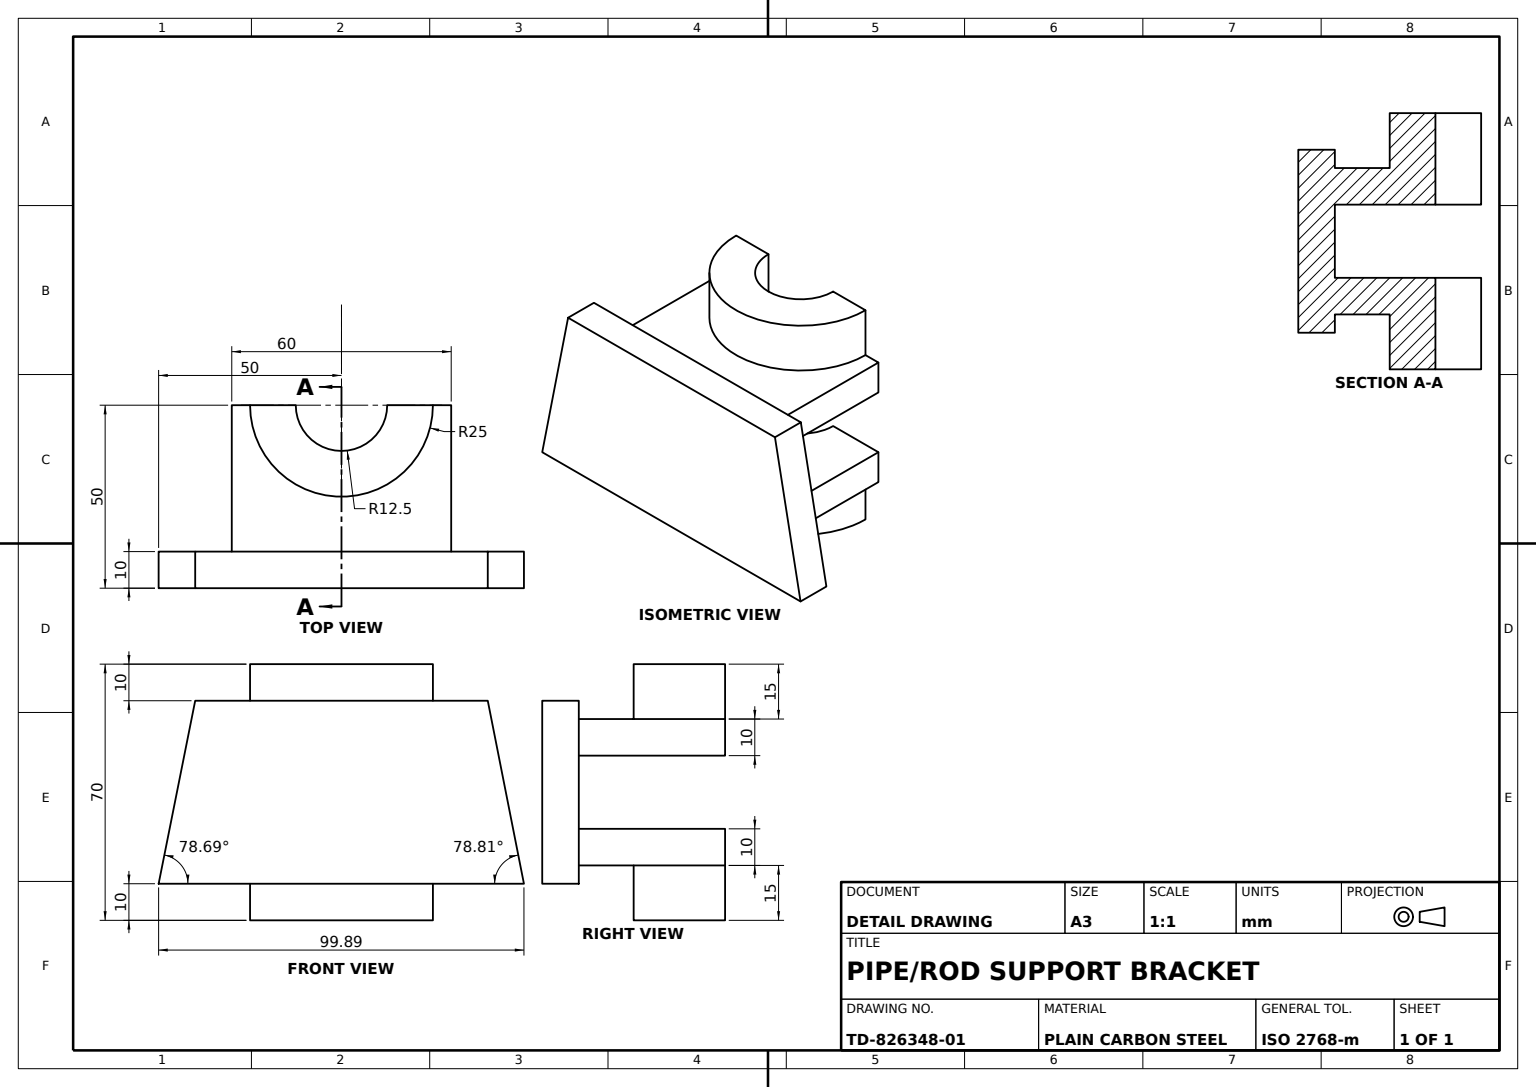
SolidWorks part; units mm, degrees
material "Plain Carbon Steel"
ref_plane "Front Plane" through (0, 0, 0) normal (0, 0, 1) x (1, 0, 0)
ref_plane "Top Plane" through (0, 0, 0) normal (0, 1, 0) x (1, 0, 0)
ref_plane "Right Plane" through (0, 0, 0) normal (1, 0, 0) x (0, 0, -1)
sketch "Base Plate Sketch" plane through (0, 0, 0) normal (0, 0, 1) x (1, 0, 0)
  line L0 (0, 0) -> (100, 0)
  line L1 (100, 0) -> (100, 50)
  line L2 (100, 50) -> (0, 50)
  line L3 (0, 50) -> (0, 0)
  dimension "D1" = 100
  dimension "D2" = 50
extrude "Base Plate 10mm" add sketch "Base Plate Sketch" along normal blind 10
ref_plane "Plane3" through (0, 0, 10) normal (0, 0, 1) x (1, 0, 0)
ref_plane "Plane4" through (50, 0, 0) normal (1, 0, 0) x (0, 0, -1)
ref_plane "Plane5" through (0, 50, 0) normal (0, 1, 0) x (1, 0, 0)
ref_plane "Arm Plane Offset 45mm" through (0, 45, 0) normal (0, 1, 0) x (1, 0, 0)
sketch "Support Arm Sketch" plane through (0, 45, 0) normal (0, 1, 0) x (1, 0, 0)
  line L0 (50, 0) -> (20, 0)
  line L1 (100, 0) -> (0, 0) construction
  line L2 (20, 0) -> (20, 40)
  line L3 (20, 40) -> (80, 40)
  line L4 (80, 40) -> (80, 0)
  line L5 (80, 0) -> (50, 0)
  dimension "D1" = 30
  dimension "D2" = 40
extrude "Support Arm" add sketch "Support Arm Sketch" against normal blind 10
ref_plane "Arm Mirror Plane" through (0, 25, 0) normal (0, 1, 0) x (1, 0, 0)
mirror "Support Arm Mirror" about plane through (0, 25, 0) normal (0, 1, 0) of "Support Arm"
sketch "Arm Relief Cut Sketch" plane through (0, 45, 0) normal (0, 1, 0) x (1, 0, 0)
  line L0 (80, 40) -> (20, 40) construction
  circle A0 centre (50, 40) radius 12.5
  dimension "D1" = 25
extrude "Arm Relief Cut" cut sketch "Arm Relief Cut Sketch" against normal through all
sketch "Bearing Seat Boss Sketch" plane through (0, 45, 0) normal (0, 1, 0) x (1, 0, 0)
  line L1 (25, 40) -> (37.5, 40)
  line L2 (62.5, 40) -> (75, 40)
  arc A1 (37.5, 40) -> (62.5, 40) centre (50, 40) ccw
  arc A2 (25, 40) -> (75, 40) centre (50, 40) ccw
extrude "Bearing Seat Boss 15mm" add sketch "Bearing Seat Boss Sketch" along normal blind 15
mirror "Bearing Seat Boss Mirror" about plane through (0, 25, 0) normal (0, 1, 0) of "Bearing Seat Boss 15mm"
sketch "Plate Taper Cut Sketch" plane through (0, 0, 0) normal (0, 0, -1) x (-1, 0, 0)
  line L0 (-100, 50) -> (-90, 50)
  line L1 (-100, 50) -> (0, 50) construction
  line L2 (-90, 50) -> (-100, -0.5529)
  line L3 (-100, -0.5529) -> (-100, 50)
  line L4 (0, 50) -> (-10, 50)
  line L5 (-10, 50) -> (0, 0)
  line L6 (0, 0) -> (0, 50)
  line L7 (-20, 15) -> (-20, 5) construction
  line L8 (-20, 5) -> (-80, 5) construction
  dimension "D1" = 10
  dimension "D2" = 5.5529
extrude "Plate Taper Cut" cut sketch "Plate Taper Cut Sketch" against normal blind 15
